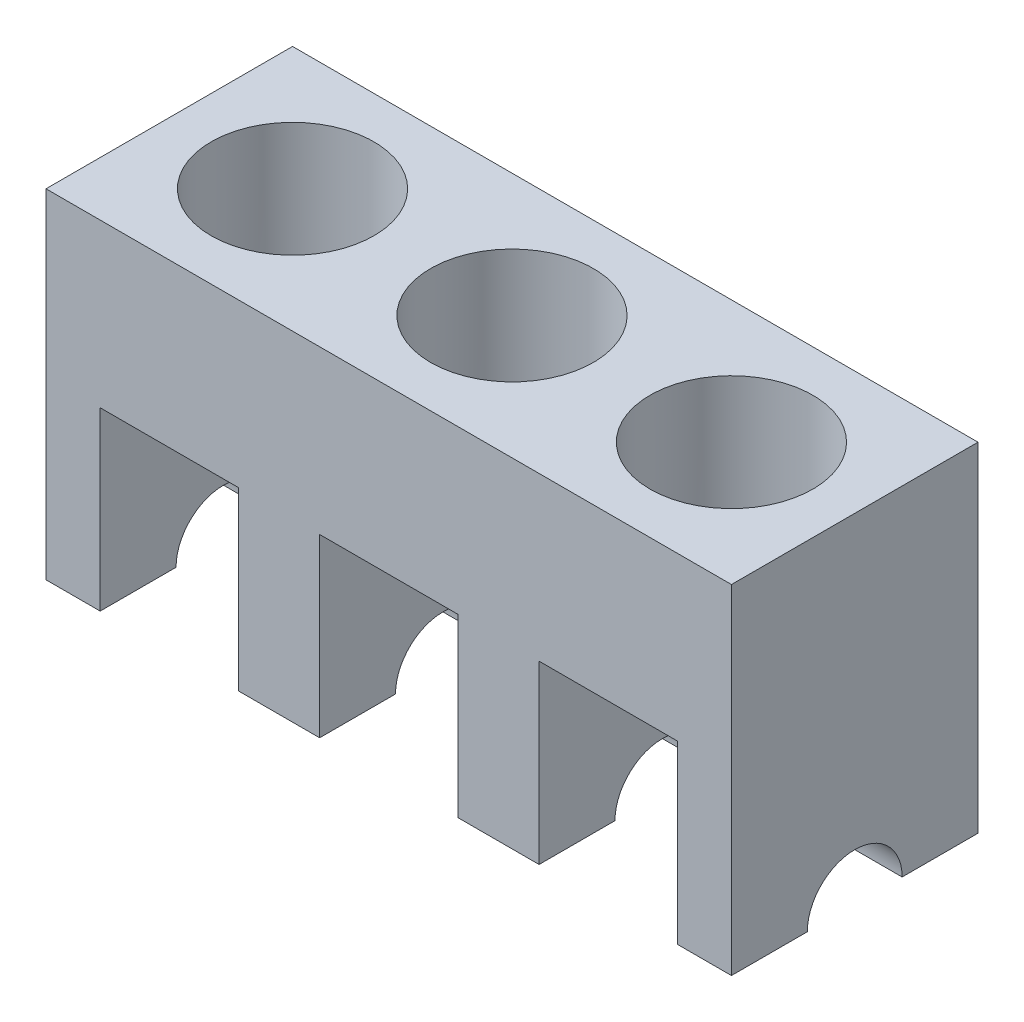
ISO-10303-21;
HEADER;
FILE_DESCRIPTION(('STEP AP214'),'2;1');
FILE_NAME('part.step','',(''),(''),'','','');
FILE_SCHEMA(('AUTOMOTIVE_DESIGN { 1 0 10303 214 1 1 1 1 }'));
ENDSEC;
DATA;
#1=APPLICATION_CONTEXT('core data for automotive mechanical design processes');
#2=APPLICATION_PROTOCOL_DEFINITION('international standard','automotive_design',2000,#1);
#3=PRODUCT_CONTEXT('',#1,'mechanical');
#4=PRODUCT('Part','Part','',(#3));
#5=PRODUCT_RELATED_PRODUCT_CATEGORY('part','',(#4));
#6=PRODUCT_DEFINITION_FORMATION('','',#4);
#7=PRODUCT_DEFINITION_CONTEXT('part definition',#1,'design');
#8=PRODUCT_DEFINITION('design','',#6,#7);
#9=PRODUCT_DEFINITION_SHAPE('','',#8);
#10=(LENGTH_UNIT() NAMED_UNIT(*) SI_UNIT(.MILLI.,.METRE.));
#11=(NAMED_UNIT(*) PLANE_ANGLE_UNIT() SI_UNIT($,.RADIAN.));
#12=(NAMED_UNIT(*) SI_UNIT($,.STERADIAN.) SOLID_ANGLE_UNIT());
#13=UNCERTAINTY_MEASURE_WITH_UNIT(LENGTH_MEASURE(1.E-05),#10,'distance_accuracy_value','');
#14=(GEOMETRIC_REPRESENTATION_CONTEXT(3) GLOBAL_UNCERTAINTY_ASSIGNED_CONTEXT((#13)) GLOBAL_UNIT_ASSIGNED_CONTEXT((#10,
#11,#12)) REPRESENTATION_CONTEXT('',''));
#15=CARTESIAN_POINT('',(0.,0.,0.));
#16=DIRECTION('',(0.,0.,1.));
#17=DIRECTION('',(1.,0.,0.));
#18=AXIS2_PLACEMENT_3D('',#15,#16,#17);
#19=CARTESIAN_POINT('',(-106.5,2.5,45.5));
#20=DIRECTION('',(0.,1.,0.));
#21=DIRECTION('',(-1.,0.,0.));
#22=AXIS2_PLACEMENT_3D('',#19,#20,#21);
#23=PLANE('',#22);
#24=DIRECTION('',(0.,0.,-1.));
#25=VECTOR('',#24,1.);
#26=CARTESIAN_POINT('',(-106.5,2.5,45.5));
#27=LINE('',#26,#25);
#28=CARTESIAN_POINT('',(-106.5,2.5,45.5));
#29=VERTEX_POINT('',#28);
#30=CARTESIAN_POINT('',(-106.5,2.5,15.8981917210732));
#31=VERTEX_POINT('',#30);
#32=EDGE_CURVE('E322',#29,#31,#27,.T.);
#33=ORIENTED_EDGE('',*,*,#32,.T.);
#34=CARTESIAN_POINT('',(-80.9999999999999,2.5,0.));
#35=DIRECTION('',(0.,1.,0.));
#36=DIRECTION('',(-1.,0.,0.));
#37=AXIS2_PLACEMENT_3D('',#34,#35,#36);
#38=CIRCLE('',#37,30.05);
#39=CARTESIAN_POINT('',(-55.4999999999999,2.5,15.8981917210731));
#40=VERTEX_POINT('',#39);
#41=EDGE_CURVE('E318',#31,#40,#38,.T.);
#42=ORIENTED_EDGE('',*,*,#41,.T.);
#43=DIRECTION('',(0.,0.,-1.));
#44=VECTOR('',#43,1.);
#45=CARTESIAN_POINT('',(-55.4999999999999,2.5,45.5));
#46=LINE('',#45,#44);
#47=CARTESIAN_POINT('',(-55.4999999999999,2.5,45.5));
#48=VERTEX_POINT('',#47);
#49=EDGE_CURVE('E314',#48,#40,#46,.T.);
#50=ORIENTED_EDGE('',*,*,#49,.F.);
#51=DIRECTION('',(1.,0.,0.));
#52=VECTOR('',#51,1.);
#53=CARTESIAN_POINT('',(-106.5,2.5,45.5));
#54=LINE('',#53,#52);
#55=EDGE_CURVE('E397',#29,#48,#54,.T.);
#56=ORIENTED_EDGE('',*,*,#55,.F.);
#57=EDGE_LOOP('',(#33,#42,#50,#56));
#58=FACE_BOUND('',#57,.T.);
#59=ADVANCED_FACE('F39',(#58),#23,.F.);
#60=CARTESIAN_POINT('',(-25.4999999999999,2.5,45.5));
#61=DIRECTION('',(0.,1.,0.));
#62=DIRECTION('',(0.,0.,1.));
#63=AXIS2_PLACEMENT_3D('',#60,#61,#62);
#64=PLANE('',#63);
#65=DIRECTION('',(0.,0.,-1.));
#66=VECTOR('',#65,1.);
#67=CARTESIAN_POINT('',(25.5000000000001,2.5,45.5));
#68=LINE('',#67,#66);
#69=CARTESIAN_POINT('',(25.5000000000001,2.5,-15.898191721073));
#70=VERTEX_POINT('',#69);
#71=CARTESIAN_POINT('',(25.5000000000001,2.5,-45.5));
#72=VERTEX_POINT('',#71);
#73=EDGE_CURVE('E484',#70,#72,#68,.T.);
#74=ORIENTED_EDGE('',*,*,#73,.F.);
#75=CARTESIAN_POINT('',(0.,2.5,0.));
#76=DIRECTION('',(0.,1.,0.));
#77=DIRECTION('',(0.,0.,1.));
#78=AXIS2_PLACEMENT_3D('',#75,#76,#77);
#79=CIRCLE('',#78,30.05);
#80=CARTESIAN_POINT('',(-25.4999999999999,2.5,-15.8981917210733));
#81=VERTEX_POINT('',#80);
#82=EDGE_CURVE('E617',#70,#81,#79,.T.);
#83=ORIENTED_EDGE('',*,*,#82,.T.);
#84=DIRECTION('',(0.,0.,-1.));
#85=VECTOR('',#84,1.);
#86=CARTESIAN_POINT('',(-25.4999999999999,2.5,45.5));
#87=LINE('',#86,#85);
#88=CARTESIAN_POINT('',(-25.4999999999999,2.5,-45.5));
#89=VERTEX_POINT('',#88);
#90=EDGE_CURVE('E487',#81,#89,#87,.T.);
#91=ORIENTED_EDGE('',*,*,#90,.T.);
#92=DIRECTION('',(1.,0.,0.));
#93=VECTOR('',#92,1.);
#94=CARTESIAN_POINT('',(-25.4999999999999,2.5,-45.5));
#95=LINE('',#94,#93);
#96=EDGE_CURVE('E441',#89,#72,#95,.T.);
#97=ORIENTED_EDGE('',*,*,#96,.T.);
#98=EDGE_LOOP('',(#74,#83,#91,#97));
#99=FACE_BOUND('',#98,.T.);
#100=ADVANCED_FACE('F621',(#99),#64,.F.);
#101=CARTESIAN_POINT('',(55.5000000000001,2.5,45.5));
#102=DIRECTION('',(0.,1.,0.));
#103=DIRECTION('',(0.,0.,1.));
#104=AXIS2_PLACEMENT_3D('',#101,#102,#103);
#105=PLANE('',#104);
#106=DIRECTION('',(0.,0.,-1.));
#107=VECTOR('',#106,1.);
#108=CARTESIAN_POINT('',(106.5,2.5,45.5));
#109=LINE('',#108,#107);
#110=CARTESIAN_POINT('',(106.5,2.5,-15.8981917210732));
#111=VERTEX_POINT('',#110);
#112=CARTESIAN_POINT('',(106.5,2.5,-45.5));
#113=VERTEX_POINT('',#112);
#114=EDGE_CURVE('E473',#111,#113,#109,.T.);
#115=ORIENTED_EDGE('',*,*,#114,.F.);
#116=CARTESIAN_POINT('',(81.0000000000001,2.5,0.));
#117=DIRECTION('',(0.,1.,0.));
#118=DIRECTION('',(0.,0.,1.));
#119=AXIS2_PLACEMENT_3D('',#116,#117,#118);
#120=CIRCLE('',#119,30.05);
#121=CARTESIAN_POINT('',(55.5000000000001,2.5,-15.8981917210732));
#122=VERTEX_POINT('',#121);
#123=EDGE_CURVE('E601',#111,#122,#120,.T.);
#124=ORIENTED_EDGE('',*,*,#123,.T.);
#125=DIRECTION('',(0.,0.,-1.));
#126=VECTOR('',#125,1.);
#127=CARTESIAN_POINT('',(55.5000000000001,2.5,45.5));
#128=LINE('',#127,#126);
#129=CARTESIAN_POINT('',(55.5000000000001,2.5,-45.5));
#130=VERTEX_POINT('',#129);
#131=EDGE_CURVE('E471',#122,#130,#128,.T.);
#132=ORIENTED_EDGE('',*,*,#131,.T.);
#133=DIRECTION('',(1.,0.,0.));
#134=VECTOR('',#133,1.);
#135=CARTESIAN_POINT('',(55.5000000000001,2.5,-45.5));
#136=LINE('',#135,#134);
#137=EDGE_CURVE('E457',#130,#113,#136,.T.);
#138=ORIENTED_EDGE('',*,*,#137,.T.);
#139=EDGE_LOOP('',(#115,#124,#132,#138));
#140=FACE_BOUND('',#139,.T.);
#141=ADVANCED_FACE('F655',(#140),#105,.F.);
#142=CARTESIAN_POINT('',(-126.5,-62.5,45.5));
#143=DIRECTION('',(0.,1.,0.));
#144=DIRECTION('',(0.,0.,1.));
#145=AXIS2_PLACEMENT_3D('',#142,#143,#144);
#146=PLANE('',#145);
#147=DIRECTION('',(0.,0.,-1.));
#148=VECTOR('',#147,1.);
#149=CARTESIAN_POINT('',(-126.5,-62.5,45.5));
#150=LINE('',#149,#148);
#151=CARTESIAN_POINT('',(-126.5,-62.5,45.5));
#152=VERTEX_POINT('',#151);
#153=CARTESIAN_POINT('',(-126.5,-62.5,17.5));
#154=VERTEX_POINT('',#153);
#155=EDGE_CURVE('E508',#152,#154,#150,.T.);
#156=ORIENTED_EDGE('',*,*,#155,.T.);
#157=DIRECTION('',(1.,0.,0.));
#158=VECTOR('',#157,1.);
#159=CARTESIAN_POINT('',(-126.5,-62.5,17.5));
#160=LINE('',#159,#158);
#161=CARTESIAN_POINT('',(-106.5,-62.5,17.5));
#162=VERTEX_POINT('',#161);
#163=EDGE_CURVE('E379',#154,#162,#160,.T.);
#164=ORIENTED_EDGE('',*,*,#163,.T.);
#165=DIRECTION('',(0.,0.,-1.));
#166=VECTOR('',#165,1.);
#167=CARTESIAN_POINT('',(-106.5,-62.5,45.5));
#168=LINE('',#167,#166);
#169=CARTESIAN_POINT('',(-106.5,-62.5,45.5));
#170=VERTEX_POINT('',#169);
#171=EDGE_CURVE('E507',#170,#162,#168,.T.);
#172=ORIENTED_EDGE('',*,*,#171,.F.);
#173=DIRECTION('',(1.,0.,0.));
#174=VECTOR('',#173,1.);
#175=CARTESIAN_POINT('',(-126.5,-62.5,45.5));
#176=LINE('',#175,#174);
#177=EDGE_CURVE('E395',#152,#170,#176,.T.);
#178=ORIENTED_EDGE('',*,*,#177,.F.);
#179=EDGE_LOOP('',(#156,#164,#172,#178));
#180=FACE_BOUND('',#179,.T.);
#181=ADVANCED_FACE('F558',(#180),#146,.F.);
#182=CARTESIAN_POINT('',(-55.4999999999999,-62.5,45.5));
#183=DIRECTION('',(0.,1.,0.));
#184=DIRECTION('',(-1.,0.,0.));
#185=AXIS2_PLACEMENT_3D('',#182,#183,#184);
#186=PLANE('',#185);
#187=DIRECTION('',(0.,0.,-1.));
#188=VECTOR('',#187,1.);
#189=CARTESIAN_POINT('',(-55.4999999999999,-62.5,45.5));
#190=LINE('',#189,#188);
#191=CARTESIAN_POINT('',(-55.4999999999999,-62.5,45.5));
#192=VERTEX_POINT('',#191);
#193=CARTESIAN_POINT('',(-55.4999999999999,-62.5,17.5));
#194=VERTEX_POINT('',#193);
#195=EDGE_CURVE('E499',#192,#194,#190,.T.);
#196=ORIENTED_EDGE('',*,*,#195,.T.);
#197=DIRECTION('',(1.,0.,0.));
#198=VECTOR('',#197,1.);
#199=CARTESIAN_POINT('',(-126.5,-62.5,17.5));
#200=LINE('',#199,#198);
#201=CARTESIAN_POINT('',(-25.4999999999999,-62.5,17.5));
#202=VERTEX_POINT('',#201);
#203=EDGE_CURVE('E366',#194,#202,#200,.T.);
#204=ORIENTED_EDGE('',*,*,#203,.T.);
#205=DIRECTION('',(0.,0.,-1.));
#206=VECTOR('',#205,1.);
#207=CARTESIAN_POINT('',(-25.4999999999999,-62.5,45.5));
#208=LINE('',#207,#206);
#209=CARTESIAN_POINT('',(-25.4999999999999,-62.5,45.5));
#210=VERTEX_POINT('',#209);
#211=EDGE_CURVE('E493',#210,#202,#208,.T.);
#212=ORIENTED_EDGE('',*,*,#211,.F.);
#213=DIRECTION('',(1.,0.,0.));
#214=VECTOR('',#213,1.);
#215=CARTESIAN_POINT('',(-55.4999999999999,-62.5,45.5));
#216=LINE('',#215,#214);
#217=EDGE_CURVE('E398',#192,#210,#216,.T.);
#218=ORIENTED_EDGE('',*,*,#217,.F.);
#219=EDGE_LOOP('',(#196,#204,#212,#218));
#220=FACE_BOUND('',#219,.T.);
#221=ADVANCED_FACE('F567',(#220),#186,.F.);
#222=CARTESIAN_POINT('',(25.5000000000001,-62.5,45.5));
#223=DIRECTION('',(0.,1.,0.));
#224=DIRECTION('',(0.,0.,1.));
#225=AXIS2_PLACEMENT_3D('',#222,#223,#224);
#226=PLANE('',#225);
#227=DIRECTION('',(0.,0.,-1.));
#228=VECTOR('',#227,1.);
#229=CARTESIAN_POINT('',(25.5000000000001,-62.5,45.5));
#230=LINE('',#229,#228);
#231=CARTESIAN_POINT('',(25.5000000000001,-62.5,45.5));
#232=VERTEX_POINT('',#231);
#233=CARTESIAN_POINT('',(25.5000000000001,-62.5,17.5));
#234=VERTEX_POINT('',#233);
#235=EDGE_CURVE('E485',#232,#234,#230,.T.);
#236=ORIENTED_EDGE('',*,*,#235,.T.);
#237=DIRECTION('',(1.,0.,0.));
#238=VECTOR('',#237,1.);
#239=CARTESIAN_POINT('',(-126.5,-62.5,17.5));
#240=LINE('',#239,#238);
#241=CARTESIAN_POINT('',(55.5000000000001,-62.5,17.5));
#242=VERTEX_POINT('',#241);
#243=EDGE_CURVE('E357',#234,#242,#240,.T.);
#244=ORIENTED_EDGE('',*,*,#243,.T.);
#245=DIRECTION('',(0.,0.,-1.));
#246=VECTOR('',#245,1.);
#247=CARTESIAN_POINT('',(55.5000000000001,-62.5,45.5));
#248=LINE('',#247,#246);
#249=CARTESIAN_POINT('',(55.5000000000001,-62.5,45.5));
#250=VERTEX_POINT('',#249);
#251=EDGE_CURVE('E476',#250,#242,#248,.T.);
#252=ORIENTED_EDGE('',*,*,#251,.F.);
#253=DIRECTION('',(1.,0.,0.));
#254=VECTOR('',#253,1.);
#255=CARTESIAN_POINT('',(25.5000000000001,-62.5,45.5));
#256=LINE('',#255,#254);
#257=EDGE_CURVE('E407',#232,#250,#256,.T.);
#258=ORIENTED_EDGE('',*,*,#257,.F.);
#259=EDGE_LOOP('',(#236,#244,#252,#258));
#260=FACE_BOUND('',#259,.T.);
#261=ADVANCED_FACE('F586',(#260),#226,.F.);
#262=CARTESIAN_POINT('',(106.5,-62.5,45.5));
#263=DIRECTION('',(0.,1.,0.));
#264=DIRECTION('',(0.,0.,1.));
#265=AXIS2_PLACEMENT_3D('',#262,#263,#264);
#266=PLANE('',#265);
#267=DIRECTION('',(0.,0.,-1.));
#268=VECTOR('',#267,1.);
#269=CARTESIAN_POINT('',(106.5,-62.5,45.5));
#270=LINE('',#269,#268);
#271=CARTESIAN_POINT('',(106.5,-62.5,45.5));
#272=VERTEX_POINT('',#271);
#273=CARTESIAN_POINT('',(106.5,-62.5,17.5));
#274=VERTEX_POINT('',#273);
#275=EDGE_CURVE('E469',#272,#274,#270,.T.);
#276=ORIENTED_EDGE('',*,*,#275,.T.);
#277=DIRECTION('',(1.,0.,0.));
#278=VECTOR('',#277,1.);
#279=CARTESIAN_POINT('',(-126.5,-62.5,17.5));
#280=LINE('',#279,#278);
#281=CARTESIAN_POINT('',(126.5,-62.5,17.5));
#282=VERTEX_POINT('',#281);
#283=EDGE_CURVE('E278',#274,#282,#280,.T.);
#284=ORIENTED_EDGE('',*,*,#283,.T.);
#285=DIRECTION('',(0.,0.,-1.));
#286=VECTOR('',#285,1.);
#287=CARTESIAN_POINT('',(126.5,-62.5,45.5));
#288=LINE('',#287,#286);
#289=CARTESIAN_POINT('',(126.5,-62.5,45.5));
#290=VERTEX_POINT('',#289);
#291=EDGE_CURVE('E463',#290,#282,#288,.T.);
#292=ORIENTED_EDGE('',*,*,#291,.F.);
#293=DIRECTION('',(1.,0.,0.));
#294=VECTOR('',#293,1.);
#295=CARTESIAN_POINT('',(106.5,-62.5,45.5));
#296=LINE('',#295,#294);
#297=EDGE_CURVE('E418',#272,#290,#296,.T.);
#298=ORIENTED_EDGE('',*,*,#297,.F.);
#299=EDGE_LOOP('',(#276,#284,#292,#298));
#300=FACE_BOUND('',#299,.T.);
#301=ADVANCED_FACE('F521',(#300),#266,.F.);
#302=CARTESIAN_POINT('',(126.5,-62.5,45.5));
#303=DIRECTION('',(-1.,0.,0.));
#304=DIRECTION('',(0.,0.,1.));
#305=AXIS2_PLACEMENT_3D('',#302,#303,#304);
#306=PLANE('',#305);
#307=ORIENTED_EDGE('',*,*,#291,.T.);
#308=CARTESIAN_POINT('',(126.5,-62.5,0.));
#309=DIRECTION('',(1.,0.,0.));
#310=DIRECTION('',(0.,0.,-1.));
#311=AXIS2_PLACEMENT_3D('',#308,#309,#310);
#312=CIRCLE('',#311,17.5);
#313=CARTESIAN_POINT('',(126.5,-62.5,-17.5));
#314=VERTEX_POINT('',#313);
#315=EDGE_CURVE('E337',#314,#282,#312,.T.);
#316=ORIENTED_EDGE('',*,*,#315,.F.);
#317=CARTESIAN_POINT('',(126.5,-62.5,-45.5));
#318=VERTEX_POINT('',#317);
#319=EDGE_CURVE('E416',#314,#318,#288,.T.);
#320=ORIENTED_EDGE('',*,*,#319,.T.);
#321=DIRECTION('',(0.,1.,0.));
#322=VECTOR('',#321,1.);
#323=CARTESIAN_POINT('',(126.5,-62.5,-45.5));
#324=LINE('',#323,#322);
#325=CARTESIAN_POINT('',(126.5,62.5,-45.5));
#326=VERTEX_POINT('',#325);
#327=EDGE_CURVE('E382',#318,#326,#324,.T.);
#328=ORIENTED_EDGE('',*,*,#327,.T.);
#329=DIRECTION('',(0.,0.,-1.));
#330=VECTOR('',#329,1.);
#331=CARTESIAN_POINT('',(126.5,62.5,45.5));
#332=LINE('',#331,#330);
#333=CARTESIAN_POINT('',(126.5,62.5,45.5));
#334=VERTEX_POINT('',#333);
#335=EDGE_CURVE('E516',#334,#326,#332,.T.);
#336=ORIENTED_EDGE('',*,*,#335,.F.);
#337=DIRECTION('',(0.,1.,0.));
#338=VECTOR('',#337,1.);
#339=CARTESIAN_POINT('',(126.5,-62.5,45.5));
#340=LINE('',#339,#338);
#341=EDGE_CURVE('E383',#290,#334,#340,.T.);
#342=ORIENTED_EDGE('',*,*,#341,.F.);
#343=EDGE_LOOP('',(#307,#316,#320,#328,#336,#342));
#344=FACE_BOUND('',#343,.T.);
#345=ADVANCED_FACE('F41',(#344),#306,.F.);
#346=CARTESIAN_POINT('',(-126.5,62.5,45.5));
#347=DIRECTION('',(0.,-1.,0.));
#348=DIRECTION('',(0.,0.,-1.));
#349=AXIS2_PLACEMENT_3D('',#346,#347,#348);
#350=PLANE('',#349);
#351=CARTESIAN_POINT('',(-80.9999999999999,62.5,0.));
#352=DIRECTION('',(0.,1.,0.));
#353=DIRECTION('',(0.,0.,1.));
#354=AXIS2_PLACEMENT_3D('',#351,#352,#353);
#355=CIRCLE('',#354,30.05);
#356=CARTESIAN_POINT('',(-80.9999999999999,62.5,30.05));
#357=VERTEX_POINT('',#356);
#358=EDGE_CURVE('E634',#357,#357,#355,.T.);
#359=ORIENTED_EDGE('',*,*,#358,.F.);
#360=EDGE_LOOP('',(#359));
#361=FACE_BOUND('',#360,.T.);
#362=CARTESIAN_POINT('',(0.,62.5,0.));
#363=DIRECTION('',(0.,1.,0.));
#364=DIRECTION('',(0.,0.,1.));
#365=AXIS2_PLACEMENT_3D('',#362,#363,#364);
#366=CIRCLE('',#365,30.05);
#367=CARTESIAN_POINT('',(0.,62.5,30.05));
#368=VERTEX_POINT('',#367);
#369=EDGE_CURVE('E287',#368,#368,#366,.T.);
#370=ORIENTED_EDGE('',*,*,#369,.F.);
#371=EDGE_LOOP('',(#370));
#372=FACE_BOUND('',#371,.T.);
#373=CARTESIAN_POINT('',(81.0000000000001,62.5,0.));
#374=DIRECTION('',(0.,1.,0.));
#375=DIRECTION('',(0.,0.,1.));
#376=AXIS2_PLACEMENT_3D('',#373,#374,#375);
#377=CIRCLE('',#376,30.05);
#378=CARTESIAN_POINT('',(81.0000000000001,62.5,30.05));
#379=VERTEX_POINT('',#378);
#380=EDGE_CURVE('E644',#379,#379,#377,.T.);
#381=ORIENTED_EDGE('',*,*,#380,.F.);
#382=EDGE_LOOP('',(#381));
#383=FACE_BOUND('',#382,.T.);
#384=DIRECTION('',(-1.,0.,0.));
#385=VECTOR('',#384,1.);
#386=CARTESIAN_POINT('',(-126.5,62.5,-45.5));
#387=LINE('',#386,#385);
#388=CARTESIAN_POINT('',(-126.5,62.5,-45.5));
#389=VERTEX_POINT('',#388);
#390=EDGE_CURVE('E423',#326,#389,#387,.T.);
#391=ORIENTED_EDGE('',*,*,#390,.T.);
#392=DIRECTION('',(0.,0.,-1.));
#393=VECTOR('',#392,1.);
#394=CARTESIAN_POINT('',(-126.5,62.5,45.5));
#395=LINE('',#394,#393);
#396=CARTESIAN_POINT('',(-126.5,62.5,45.5));
#397=VERTEX_POINT('',#396);
#398=EDGE_CURVE('E511',#397,#389,#395,.T.);
#399=ORIENTED_EDGE('',*,*,#398,.F.);
#400=DIRECTION('',(-1.,0.,0.));
#401=VECTOR('',#400,1.);
#402=CARTESIAN_POINT('',(-126.5,62.5,45.5));
#403=LINE('',#402,#401);
#404=EDGE_CURVE('E390',#334,#397,#403,.T.);
#405=ORIENTED_EDGE('',*,*,#404,.F.);
#406=ORIENTED_EDGE('',*,*,#335,.T.);
#407=EDGE_LOOP('',(#391,#399,#405,#406));
#408=FACE_BOUND('',#407,.T.);
#409=ADVANCED_FACE('F548',(#361,#372,#383,#408),#350,.F.);
#410=CARTESIAN_POINT('',(-126.5,-62.5,45.5));
#411=DIRECTION('',(1.,0.,0.));
#412=DIRECTION('',(0.,0.,-1.));
#413=AXIS2_PLACEMENT_3D('',#410,#411,#412);
#414=PLANE('',#413);
#415=CARTESIAN_POINT('',(-126.5,-62.5,-17.5));
#416=VERTEX_POINT('',#415);
#417=CARTESIAN_POINT('',(-126.5,-62.5,-45.5));
#418=VERTEX_POINT('',#417);
#419=EDGE_CURVE('E506',#416,#418,#150,.T.);
#420=ORIENTED_EDGE('',*,*,#419,.F.);
#421=CARTESIAN_POINT('',(-126.5,-62.5,0.));
#422=DIRECTION('',(1.,0.,0.));
#423=DIRECTION('',(0.,0.,-1.));
#424=AXIS2_PLACEMENT_3D('',#421,#422,#423);
#425=CIRCLE('',#424,17.5);
#426=EDGE_CURVE('E345',#416,#154,#425,.T.);
#427=ORIENTED_EDGE('',*,*,#426,.T.);
#428=ORIENTED_EDGE('',*,*,#155,.F.);
#429=DIRECTION('',(0.,-1.,0.));
#430=VECTOR('',#429,1.);
#431=CARTESIAN_POINT('',(-126.5,-62.5,45.5));
#432=LINE('',#431,#430);
#433=EDGE_CURVE('E388',#397,#152,#432,.T.);
#434=ORIENTED_EDGE('',*,*,#433,.F.);
#435=ORIENTED_EDGE('',*,*,#398,.T.);
#436=DIRECTION('',(0.,-1.,0.));
#437=VECTOR('',#436,1.);
#438=CARTESIAN_POINT('',(-126.5,-62.5,-45.5));
#439=LINE('',#438,#437);
#440=EDGE_CURVE('E421',#389,#418,#439,.T.);
#441=ORIENTED_EDGE('',*,*,#440,.T.);
#442=EDGE_LOOP('',(#420,#427,#428,#434,#435,#441));
#443=FACE_BOUND('',#442,.T.);
#444=ADVANCED_FACE('F551',(#443),#414,.F.);
#445=CARTESIAN_POINT('',(-106.5,-62.5,-17.5));
#446=VERTEX_POINT('',#445);
#447=CARTESIAN_POINT('',(-106.5,-62.5,-45.5));
#448=VERTEX_POINT('',#447);
#449=EDGE_CURVE('E504',#446,#448,#168,.T.);
#450=ORIENTED_EDGE('',*,*,#449,.F.);
#451=DIRECTION('',(1.,0.,0.));
#452=VECTOR('',#451,1.);
#453=CARTESIAN_POINT('',(-126.5,-62.5,-17.5));
#454=LINE('',#453,#452);
#455=EDGE_CURVE('E380',#446,#416,#454,.F.);
#456=ORIENTED_EDGE('',*,*,#455,.T.);
#457=ORIENTED_EDGE('',*,*,#419,.T.);
#458=DIRECTION('',(1.,0.,0.));
#459=VECTOR('',#458,1.);
#460=CARTESIAN_POINT('',(-126.5,-62.5,-45.5));
#461=LINE('',#460,#459);
#462=EDGE_CURVE('E426',#418,#448,#461,.T.);
#463=ORIENTED_EDGE('',*,*,#462,.T.);
#464=EDGE_LOOP('',(#450,#456,#457,#463));
#465=FACE_BOUND('',#464,.T.);
#466=ADVANCED_FACE('F687',(#465),#146,.F.);
#467=CARTESIAN_POINT('',(-106.5,-62.5,45.5));
#468=DIRECTION('',(-1.,0.,0.));
#469=DIRECTION('',(0.,-1.,0.));
#470=AXIS2_PLACEMENT_3D('',#467,#468,#469);
#471=PLANE('',#470);
#472=DIRECTION('',(0.,0.,-1.));
#473=VECTOR('',#472,1.);
#474=CARTESIAN_POINT('',(-106.5,-18.5,45.5));
#475=LINE('',#474,#473);
#476=CARTESIAN_POINT('',(-106.5,-18.5,15.8981917210732));
#477=VERTEX_POINT('',#476);
#478=CARTESIAN_POINT('',(-106.5,-18.5,-15.8981917210732));
#479=VERTEX_POINT('',#478);
#480=EDGE_CURVE('E326',#477,#479,#475,.T.);
#481=ORIENTED_EDGE('',*,*,#480,.F.);
#482=DIRECTION('',(0.,1.,0.));
#483=VECTOR('',#482,1.);
#484=CARTESIAN_POINT('',(-106.5,-18.5,15.8981917210732));
#485=LINE('',#484,#483);
#486=EDGE_CURVE('E324',#477,#31,#485,.T.);
#487=ORIENTED_EDGE('',*,*,#486,.T.);
#488=ORIENTED_EDGE('',*,*,#32,.F.);
#489=DIRECTION('',(0.,1.,0.));
#490=VECTOR('',#489,1.);
#491=CARTESIAN_POINT('',(-106.5,-62.5,45.5));
#492=LINE('',#491,#490);
#493=EDGE_CURVE('E393',#170,#29,#492,.T.);
#494=ORIENTED_EDGE('',*,*,#493,.F.);
#495=ORIENTED_EDGE('',*,*,#171,.T.);
#496=CARTESIAN_POINT('',(-106.5,-62.5,0.));
#497=DIRECTION('',(-1.,0.,0.));
#498=DIRECTION('',(0.,-1.,0.));
#499=AXIS2_PLACEMENT_3D('',#496,#497,#498);
#500=CIRCLE('',#499,17.5);
#501=EDGE_CURVE('E372',#162,#446,#500,.T.);
#502=ORIENTED_EDGE('',*,*,#501,.T.);
#503=ORIENTED_EDGE('',*,*,#449,.T.);
#504=DIRECTION('',(0.,1.,0.));
#505=VECTOR('',#504,1.);
#506=CARTESIAN_POINT('',(-106.5,-62.5,-45.5));
#507=LINE('',#506,#505);
#508=CARTESIAN_POINT('',(-106.5,2.5,-45.5));
#509=VERTEX_POINT('',#508);
#510=EDGE_CURVE('E427',#448,#509,#507,.T.);
#511=ORIENTED_EDGE('',*,*,#510,.T.);
#512=CARTESIAN_POINT('',(-106.5,2.5,-15.8981917210732));
#513=VERTEX_POINT('',#512);
#514=EDGE_CURVE('E502',#513,#509,#27,.T.);
#515=ORIENTED_EDGE('',*,*,#514,.F.);
#516=DIRECTION('',(0.,1.,0.));
#517=VECTOR('',#516,1.);
#518=CARTESIAN_POINT('',(-106.5,-18.5,-15.8981917210732));
#519=LINE('',#518,#517);
#520=EDGE_CURVE('E334',#513,#479,#519,.F.);
#521=ORIENTED_EDGE('',*,*,#520,.T.);
#522=EDGE_LOOP('',(#481,#487,#488,#494,#495,#502,#503,#511,#515,#521));
#523=FACE_BOUND('',#522,.T.);
#524=ADVANCED_FACE('F559',(#523),#471,.F.);
#525=CARTESIAN_POINT('',(-55.4999999999999,2.5,-15.8981917210731));
#526=VERTEX_POINT('',#525);
#527=CARTESIAN_POINT('',(-55.4999999999999,2.5,-45.5));
#528=VERTEX_POINT('',#527);
#529=EDGE_CURVE('E501',#526,#528,#46,.T.);
#530=ORIENTED_EDGE('',*,*,#529,.F.);
#531=EDGE_CURVE('E327',#526,#513,#38,.T.);
#532=ORIENTED_EDGE('',*,*,#531,.T.);
#533=ORIENTED_EDGE('',*,*,#514,.T.);
#534=DIRECTION('',(1.,0.,0.));
#535=VECTOR('',#534,1.);
#536=CARTESIAN_POINT('',(-106.5,2.5,-45.5));
#537=LINE('',#536,#535);
#538=EDGE_CURVE('E435',#509,#528,#537,.T.);
#539=ORIENTED_EDGE('',*,*,#538,.T.);
#540=EDGE_LOOP('',(#530,#532,#533,#539));
#541=FACE_BOUND('',#540,.T.);
#542=ADVANCED_FACE('F675',(#541),#23,.F.);
#543=CARTESIAN_POINT('',(-55.4999999999999,2.5,45.5));
#544=DIRECTION('',(1.,0.,0.));
#545=DIRECTION('',(0.,1.,0.));
#546=AXIS2_PLACEMENT_3D('',#543,#544,#545);
#547=PLANE('',#546);
#548=DIRECTION('',(0.,0.,1.));
#549=VECTOR('',#548,1.);
#550=CARTESIAN_POINT('',(-55.4999999999999,-18.5,45.5));
#551=LINE('',#550,#549);
#552=CARTESIAN_POINT('',(-55.4999999999999,-18.5,-15.8981917210731));
#553=VERTEX_POINT('',#552);
#554=CARTESIAN_POINT('',(-55.4999999999999,-18.5,15.8981917210731));
#555=VERTEX_POINT('',#554);
#556=EDGE_CURVE('E308',#553,#555,#551,.T.);
#557=ORIENTED_EDGE('',*,*,#556,.F.);
#558=DIRECTION('',(0.,1.,0.));
#559=VECTOR('',#558,1.);
#560=CARTESIAN_POINT('',(-55.4999999999999,-18.5,-15.8981917210731));
#561=LINE('',#560,#559);
#562=EDGE_CURVE('E11',#553,#526,#561,.T.);
#563=ORIENTED_EDGE('',*,*,#562,.T.);
#564=ORIENTED_EDGE('',*,*,#529,.T.);
#565=DIRECTION('',(0.,-1.,0.));
#566=VECTOR('',#565,1.);
#567=CARTESIAN_POINT('',(-55.4999999999999,2.5,-45.5));
#568=LINE('',#567,#566);
#569=CARTESIAN_POINT('',(-55.4999999999999,-62.5,-45.5));
#570=VERTEX_POINT('',#569);
#571=EDGE_CURVE('E434',#528,#570,#568,.T.);
#572=ORIENTED_EDGE('',*,*,#571,.T.);
#573=CARTESIAN_POINT('',(-55.4999999999999,-62.5,-17.5));
#574=VERTEX_POINT('',#573);
#575=EDGE_CURVE('E500',#574,#570,#190,.T.);
#576=ORIENTED_EDGE('',*,*,#575,.F.);
#577=CARTESIAN_POINT('',(-55.4999999999999,-62.5,0.));
#578=DIRECTION('',(1.,0.,0.));
#579=DIRECTION('',(0.,1.,0.));
#580=AXIS2_PLACEMENT_3D('',#577,#578,#579);
#581=CIRCLE('',#580,17.5);
#582=EDGE_CURVE('E371',#574,#194,#581,.T.);
#583=ORIENTED_EDGE('',*,*,#582,.T.);
#584=ORIENTED_EDGE('',*,*,#195,.F.);
#585=DIRECTION('',(0.,-1.,0.));
#586=VECTOR('',#585,1.);
#587=CARTESIAN_POINT('',(-55.4999999999999,2.5,45.5));
#588=LINE('',#587,#586);
#589=EDGE_CURVE('E399',#48,#192,#588,.T.);
#590=ORIENTED_EDGE('',*,*,#589,.F.);
#591=ORIENTED_EDGE('',*,*,#49,.T.);
#592=DIRECTION('',(0.,1.,0.));
#593=VECTOR('',#592,1.);
#594=CARTESIAN_POINT('',(-55.4999999999999,-18.5,15.8981917210731));
#595=LINE('',#594,#593);
#596=EDGE_CURVE('E50',#40,#555,#595,.F.);
#597=ORIENTED_EDGE('',*,*,#596,.T.);
#598=EDGE_LOOP('',(#557,#563,#564,#572,#576,#583,#584,#590,#591,#597));
#599=FACE_BOUND('',#598,.T.);
#600=ADVANCED_FACE('F313',(#599),#547,.F.);
#601=CARTESIAN_POINT('',(-25.4999999999999,-62.5,-17.5));
#602=VERTEX_POINT('',#601);
#603=CARTESIAN_POINT('',(-25.4999999999999,-62.5,-45.5));
#604=VERTEX_POINT('',#603);
#605=EDGE_CURVE('E492',#602,#604,#208,.T.);
#606=ORIENTED_EDGE('',*,*,#605,.F.);
#607=DIRECTION('',(1.,0.,0.));
#608=VECTOR('',#607,1.);
#609=CARTESIAN_POINT('',(-126.5,-62.5,-17.5));
#610=LINE('',#609,#608);
#611=EDGE_CURVE('E364',#602,#574,#610,.F.);
#612=ORIENTED_EDGE('',*,*,#611,.T.);
#613=ORIENTED_EDGE('',*,*,#575,.T.);
#614=DIRECTION('',(1.,0.,0.));
#615=VECTOR('',#614,1.);
#616=CARTESIAN_POINT('',(-55.4999999999999,-62.5,-45.5));
#617=LINE('',#616,#615);
#618=EDGE_CURVE('E437',#570,#604,#617,.T.);
#619=ORIENTED_EDGE('',*,*,#618,.T.);
#620=EDGE_LOOP('',(#606,#612,#613,#619));
#621=FACE_BOUND('',#620,.T.);
#622=ADVANCED_FACE('F684',(#621),#186,.F.);
#623=CARTESIAN_POINT('',(-25.4999999999999,-62.5,45.5));
#624=DIRECTION('',(-1.,0.,0.));
#625=DIRECTION('',(0.,0.,1.));
#626=AXIS2_PLACEMENT_3D('',#623,#624,#625);
#627=PLANE('',#626);
#628=DIRECTION('',(0.,0.,-1.));
#629=VECTOR('',#628,1.);
#630=CARTESIAN_POINT('',(-25.4999999999999,-18.5,45.5));
#631=LINE('',#630,#629);
#632=CARTESIAN_POINT('',(-25.4999999999999,-18.5,15.8981917210733));
#633=VERTEX_POINT('',#632);
#634=CARTESIAN_POINT('',(-25.4999999999999,-18.5,-15.8981917210733));
#635=VERTEX_POINT('',#634);
#636=EDGE_CURVE('E608',#633,#635,#631,.T.);
#637=ORIENTED_EDGE('',*,*,#636,.F.);
#638=DIRECTION('',(0.,1.,0.));
#639=VECTOR('',#638,1.);
#640=CARTESIAN_POINT('',(-25.4999999999999,-18.5,15.8981917210733));
#641=LINE('',#640,#639);
#642=CARTESIAN_POINT('',(-25.4999999999999,2.5,15.8981917210733));
#643=VERTEX_POINT('',#642);
#644=EDGE_CURVE('E614',#633,#643,#641,.T.);
#645=ORIENTED_EDGE('',*,*,#644,.T.);
#646=CARTESIAN_POINT('',(-25.4999999999999,2.5,45.5));
#647=VERTEX_POINT('',#646);
#648=EDGE_CURVE('E489',#647,#643,#87,.T.);
#649=ORIENTED_EDGE('',*,*,#648,.F.);
#650=DIRECTION('',(0.,1.,0.));
#651=VECTOR('',#650,1.);
#652=CARTESIAN_POINT('',(-25.4999999999999,-62.5,45.5));
#653=LINE('',#652,#651);
#654=EDGE_CURVE('E405',#210,#647,#653,.T.);
#655=ORIENTED_EDGE('',*,*,#654,.F.);
#656=ORIENTED_EDGE('',*,*,#211,.T.);
#657=CARTESIAN_POINT('',(-25.4999999999999,-62.5,0.));
#658=DIRECTION('',(-1.,0.,0.));
#659=DIRECTION('',(0.,0.,1.));
#660=AXIS2_PLACEMENT_3D('',#657,#658,#659);
#661=CIRCLE('',#660,17.5);
#662=EDGE_CURVE('E362',#202,#602,#661,.T.);
#663=ORIENTED_EDGE('',*,*,#662,.T.);
#664=ORIENTED_EDGE('',*,*,#605,.T.);
#665=DIRECTION('',(0.,1.,0.));
#666=VECTOR('',#665,1.);
#667=CARTESIAN_POINT('',(-25.4999999999999,-62.5,-45.5));
#668=LINE('',#667,#666);
#669=EDGE_CURVE('E442',#604,#89,#668,.T.);
#670=ORIENTED_EDGE('',*,*,#669,.T.);
#671=ORIENTED_EDGE('',*,*,#90,.F.);
#672=DIRECTION('',(0.,1.,0.));
#673=VECTOR('',#672,1.);
#674=CARTESIAN_POINT('',(-25.4999999999999,-18.5,-15.8981917210733));
#675=LINE('',#674,#673);
#676=EDGE_CURVE('E329',#81,#635,#675,.F.);
#677=ORIENTED_EDGE('',*,*,#676,.T.);
#678=EDGE_LOOP('',(#637,#645,#649,#655,#656,#663,#664,#670,#671,#677));
#679=FACE_BOUND('',#678,.T.);
#680=ADVANCED_FACE('F571',(#679),#627,.F.);
#681=ORIENTED_EDGE('',*,*,#648,.T.);
#682=CARTESIAN_POINT('',(25.5000000000001,2.5,15.898191721073));
#683=VERTEX_POINT('',#682);
#684=EDGE_CURVE('E578',#643,#683,#79,.T.);
#685=ORIENTED_EDGE('',*,*,#684,.T.);
#686=CARTESIAN_POINT('',(25.5000000000001,2.5,45.5));
#687=VERTEX_POINT('',#686);
#688=EDGE_CURVE('E486',#687,#683,#68,.T.);
#689=ORIENTED_EDGE('',*,*,#688,.F.);
#690=DIRECTION('',(1.,0.,0.));
#691=VECTOR('',#690,1.);
#692=CARTESIAN_POINT('',(-25.4999999999999,2.5,45.5));
#693=LINE('',#692,#691);
#694=EDGE_CURVE('E404',#647,#687,#693,.T.);
#695=ORIENTED_EDGE('',*,*,#694,.F.);
#696=EDGE_LOOP('',(#681,#685,#689,#695));
#697=FACE_BOUND('',#696,.T.);
#698=ADVANCED_FACE('F576',(#697),#64,.F.);
#699=CARTESIAN_POINT('',(25.5000000000001,2.5,45.5));
#700=DIRECTION('',(1.,0.,0.));
#701=DIRECTION('',(0.,1.,0.));
#702=AXIS2_PLACEMENT_3D('',#699,#700,#701);
#703=PLANE('',#702);
#704=DIRECTION('',(0.,0.,1.));
#705=VECTOR('',#704,1.);
#706=CARTESIAN_POINT('',(25.5000000000001,-18.5,45.5));
#707=LINE('',#706,#705);
#708=CARTESIAN_POINT('',(25.5000000000001,-18.5,-15.898191721073));
#709=VERTEX_POINT('',#708);
#710=CARTESIAN_POINT('',(25.5000000000001,-18.5,15.898191721073));
#711=VERTEX_POINT('',#710);
#712=EDGE_CURVE('E293',#709,#711,#707,.T.);
#713=ORIENTED_EDGE('',*,*,#712,.F.);
#714=DIRECTION('',(0.,1.,0.));
#715=VECTOR('',#714,1.);
#716=CARTESIAN_POINT('',(25.5000000000001,-18.5,-15.898191721073));
#717=LINE('',#716,#715);
#718=EDGE_CURVE('E304',#709,#70,#717,.T.);
#719=ORIENTED_EDGE('',*,*,#718,.T.);
#720=ORIENTED_EDGE('',*,*,#73,.T.);
#721=DIRECTION('',(0.,-1.,0.));
#722=VECTOR('',#721,1.);
#723=CARTESIAN_POINT('',(25.5000000000001,2.5,-45.5));
#724=LINE('',#723,#722);
#725=CARTESIAN_POINT('',(25.5000000000001,-62.5,-45.5));
#726=VERTEX_POINT('',#725);
#727=EDGE_CURVE('E450',#72,#726,#724,.T.);
#728=ORIENTED_EDGE('',*,*,#727,.T.);
#729=CARTESIAN_POINT('',(25.5000000000001,-62.5,-17.5));
#730=VERTEX_POINT('',#729);
#731=EDGE_CURVE('E481',#730,#726,#230,.T.);
#732=ORIENTED_EDGE('',*,*,#731,.F.);
#733=CARTESIAN_POINT('',(25.5000000000001,-62.5,0.));
#734=DIRECTION('',(1.,0.,0.));
#735=DIRECTION('',(0.,1.,0.));
#736=AXIS2_PLACEMENT_3D('',#733,#734,#735);
#737=CIRCLE('',#736,17.5);
#738=EDGE_CURVE('E356',#730,#234,#737,.T.);
#739=ORIENTED_EDGE('',*,*,#738,.T.);
#740=ORIENTED_EDGE('',*,*,#235,.F.);
#741=DIRECTION('',(0.,-1.,0.));
#742=VECTOR('',#741,1.);
#743=CARTESIAN_POINT('',(25.5000000000001,2.5,45.5));
#744=LINE('',#743,#742);
#745=EDGE_CURVE('E406',#687,#232,#744,.T.);
#746=ORIENTED_EDGE('',*,*,#745,.F.);
#747=ORIENTED_EDGE('',*,*,#688,.T.);
#748=DIRECTION('',(0.,1.,0.));
#749=VECTOR('',#748,1.);
#750=CARTESIAN_POINT('',(25.5000000000001,-18.5,15.898191721073));
#751=LINE('',#750,#749);
#752=EDGE_CURVE('E299',#683,#711,#751,.F.);
#753=ORIENTED_EDGE('',*,*,#752,.T.);
#754=EDGE_LOOP('',(#713,#719,#720,#728,#732,#739,#740,#746,#747,#753));
#755=FACE_BOUND('',#754,.T.);
#756=ADVANCED_FACE('F581',(#755),#703,.F.);
#757=CARTESIAN_POINT('',(55.5000000000001,-62.5,-17.5));
#758=VERTEX_POINT('',#757);
#759=CARTESIAN_POINT('',(55.5000000000001,-62.5,-45.5));
#760=VERTEX_POINT('',#759);
#761=EDGE_CURVE('E480',#758,#760,#248,.T.);
#762=ORIENTED_EDGE('',*,*,#761,.F.);
#763=DIRECTION('',(1.,0.,0.));
#764=VECTOR('',#763,1.);
#765=CARTESIAN_POINT('',(-126.5,-62.5,-17.5));
#766=LINE('',#765,#764);
#767=EDGE_CURVE('E352',#758,#730,#766,.F.);
#768=ORIENTED_EDGE('',*,*,#767,.T.);
#769=ORIENTED_EDGE('',*,*,#731,.T.);
#770=DIRECTION('',(1.,0.,0.));
#771=VECTOR('',#770,1.);
#772=CARTESIAN_POINT('',(25.5000000000001,-62.5,-45.5));
#773=LINE('',#772,#771);
#774=EDGE_CURVE('E449',#726,#760,#773,.T.);
#775=ORIENTED_EDGE('',*,*,#774,.T.);
#776=EDGE_LOOP('',(#762,#768,#769,#775));
#777=FACE_BOUND('',#776,.T.);
#778=ADVANCED_FACE('F656',(#777),#226,.F.);
#779=CARTESIAN_POINT('',(55.5000000000001,-62.5,45.5));
#780=DIRECTION('',(-1.,0.,0.));
#781=DIRECTION('',(0.,0.,1.));
#782=AXIS2_PLACEMENT_3D('',#779,#780,#781);
#783=PLANE('',#782);
#784=DIRECTION('',(0.,0.,-1.));
#785=VECTOR('',#784,1.);
#786=CARTESIAN_POINT('',(55.5000000000001,-18.5,45.5));
#787=LINE('',#786,#785);
#788=CARTESIAN_POINT('',(55.5000000000001,-18.5,15.8981917210732));
#789=VERTEX_POINT('',#788);
#790=CARTESIAN_POINT('',(55.5000000000001,-18.5,-15.8981917210732));
#791=VERTEX_POINT('',#790);
#792=EDGE_CURVE('E597',#789,#791,#787,.T.);
#793=ORIENTED_EDGE('',*,*,#792,.F.);
#794=DIRECTION('',(0.,1.,0.));
#795=VECTOR('',#794,1.);
#796=CARTESIAN_POINT('',(55.5000000000001,-18.5,15.8981917210732));
#797=LINE('',#796,#795);
#798=CARTESIAN_POINT('',(55.5000000000001,2.5,15.8981917210732));
#799=VERTEX_POINT('',#798);
#800=EDGE_CURVE('E594',#789,#799,#797,.T.);
#801=ORIENTED_EDGE('',*,*,#800,.T.);
#802=CARTESIAN_POINT('',(55.5000000000001,2.5,45.5));
#803=VERTEX_POINT('',#802);
#804=EDGE_CURVE('E475',#803,#799,#128,.T.);
#805=ORIENTED_EDGE('',*,*,#804,.F.);
#806=DIRECTION('',(0.,1.,0.));
#807=VECTOR('',#806,1.);
#808=CARTESIAN_POINT('',(55.5000000000001,-62.5,45.5));
#809=LINE('',#808,#807);
#810=EDGE_CURVE('E409',#250,#803,#809,.T.);
#811=ORIENTED_EDGE('',*,*,#810,.F.);
#812=ORIENTED_EDGE('',*,*,#251,.T.);
#813=CARTESIAN_POINT('',(55.5000000000001,-62.5,0.));
#814=DIRECTION('',(-1.,0.,0.));
#815=DIRECTION('',(0.,0.,1.));
#816=AXIS2_PLACEMENT_3D('',#813,#814,#815);
#817=CIRCLE('',#816,17.5);
#818=EDGE_CURVE('E348',#242,#758,#817,.T.);
#819=ORIENTED_EDGE('',*,*,#818,.T.);
#820=ORIENTED_EDGE('',*,*,#761,.T.);
#821=DIRECTION('',(0.,1.,0.));
#822=VECTOR('',#821,1.);
#823=CARTESIAN_POINT('',(55.5000000000001,-62.5,-45.5));
#824=LINE('',#823,#822);
#825=EDGE_CURVE('E454',#760,#130,#824,.T.);
#826=ORIENTED_EDGE('',*,*,#825,.T.);
#827=ORIENTED_EDGE('',*,*,#131,.F.);
#828=DIRECTION('',(0.,1.,0.));
#829=VECTOR('',#828,1.);
#830=CARTESIAN_POINT('',(55.5000000000001,-18.5,-15.8981917210732));
#831=LINE('',#830,#829);
#832=EDGE_CURVE('E604',#122,#791,#831,.F.);
#833=ORIENTED_EDGE('',*,*,#832,.T.);
#834=EDGE_LOOP('',(#793,#801,#805,#811,#812,#819,#820,#826,#827,#833));
#835=FACE_BOUND('',#834,.T.);
#836=ADVANCED_FACE('F592',(#835),#783,.F.);
#837=ORIENTED_EDGE('',*,*,#804,.T.);
#838=CARTESIAN_POINT('',(106.5,2.5,15.8981917210732));
#839=VERTEX_POINT('',#838);
#840=EDGE_CURVE('E598',#799,#839,#120,.T.);
#841=ORIENTED_EDGE('',*,*,#840,.T.);
#842=CARTESIAN_POINT('',(106.5,2.5,45.5));
#843=VERTEX_POINT('',#842);
#844=EDGE_CURVE('E291',#843,#839,#109,.T.);
#845=ORIENTED_EDGE('',*,*,#844,.F.);
#846=DIRECTION('',(1.,0.,0.));
#847=VECTOR('',#846,1.);
#848=CARTESIAN_POINT('',(55.5000000000001,2.5,45.5));
#849=LINE('',#848,#847);
#850=EDGE_CURVE('E415',#803,#843,#849,.T.);
#851=ORIENTED_EDGE('',*,*,#850,.F.);
#852=EDGE_LOOP('',(#837,#841,#845,#851));
#853=FACE_BOUND('',#852,.T.);
#854=ADVANCED_FACE('F600',(#853),#105,.F.);
#855=CARTESIAN_POINT('',(106.5,2.5,45.5));
#856=DIRECTION('',(1.,0.,0.));
#857=DIRECTION('',(0.,1.,0.));
#858=AXIS2_PLACEMENT_3D('',#855,#856,#857);
#859=PLANE('',#858);
#860=DIRECTION('',(0.,0.,1.));
#861=VECTOR('',#860,1.);
#862=CARTESIAN_POINT('',(106.5,-18.5,45.5));
#863=LINE('',#862,#861);
#864=CARTESIAN_POINT('',(106.5,-18.5,-15.8981917210732));
#865=VERTEX_POINT('',#864);
#866=CARTESIAN_POINT('',(106.5,-18.5,15.8981917210732));
#867=VERTEX_POINT('',#866);
#868=EDGE_CURVE('E271',#865,#867,#863,.T.);
#869=ORIENTED_EDGE('',*,*,#868,.F.);
#870=DIRECTION('',(0.,1.,0.));
#871=VECTOR('',#870,1.);
#872=CARTESIAN_POINT('',(106.5,-18.5,-15.8981917210732));
#873=LINE('',#872,#871);
#874=EDGE_CURVE('E284',#865,#111,#873,.T.);
#875=ORIENTED_EDGE('',*,*,#874,.T.);
#876=ORIENTED_EDGE('',*,*,#114,.T.);
#877=DIRECTION('',(0.,-1.,0.));
#878=VECTOR('',#877,1.);
#879=CARTESIAN_POINT('',(106.5,2.5,-45.5));
#880=LINE('',#879,#878);
#881=CARTESIAN_POINT('',(106.5,-62.5,-45.5));
#882=VERTEX_POINT('',#881);
#883=EDGE_CURVE('E459',#113,#882,#880,.T.);
#884=ORIENTED_EDGE('',*,*,#883,.T.);
#885=CARTESIAN_POINT('',(106.5,-62.5,-17.5));
#886=VERTEX_POINT('',#885);
#887=EDGE_CURVE('E470',#886,#882,#270,.T.);
#888=ORIENTED_EDGE('',*,*,#887,.F.);
#889=CARTESIAN_POINT('',(106.5,-62.5,0.));
#890=DIRECTION('',(1.,0.,0.));
#891=DIRECTION('',(0.,1.,0.));
#892=AXIS2_PLACEMENT_3D('',#889,#890,#891);
#893=CIRCLE('',#892,17.5);
#894=EDGE_CURVE('E347',#886,#274,#893,.T.);
#895=ORIENTED_EDGE('',*,*,#894,.T.);
#896=ORIENTED_EDGE('',*,*,#275,.F.);
#897=DIRECTION('',(0.,-1.,0.));
#898=VECTOR('',#897,1.);
#899=CARTESIAN_POINT('',(106.5,2.5,45.5));
#900=LINE('',#899,#898);
#901=EDGE_CURVE('E411',#843,#272,#900,.T.);
#902=ORIENTED_EDGE('',*,*,#901,.F.);
#903=ORIENTED_EDGE('',*,*,#844,.T.);
#904=DIRECTION('',(0.,1.,0.));
#905=VECTOR('',#904,1.);
#906=CARTESIAN_POINT('',(106.5,-18.5,15.8981917210732));
#907=LINE('',#906,#905);
#908=EDGE_CURVE('E276',#839,#867,#907,.F.);
#909=ORIENTED_EDGE('',*,*,#908,.T.);
#910=EDGE_LOOP('',(#869,#875,#876,#884,#888,#895,#896,#902,#903,#909));
#911=FACE_BOUND('',#910,.T.);
#912=ADVANCED_FACE('F288',(#911),#859,.F.);
#913=ORIENTED_EDGE('',*,*,#319,.F.);
#914=DIRECTION('',(1.,0.,0.));
#915=VECTOR('',#914,1.);
#916=CARTESIAN_POINT('',(-126.5,-62.5,-17.5));
#917=LINE('',#916,#915);
#918=EDGE_CURVE('E518',#314,#886,#917,.F.);
#919=ORIENTED_EDGE('',*,*,#918,.T.);
#920=ORIENTED_EDGE('',*,*,#887,.T.);
#921=DIRECTION('',(1.,0.,0.));
#922=VECTOR('',#921,1.);
#923=CARTESIAN_POINT('',(106.5,-62.5,-45.5));
#924=LINE('',#923,#922);
#925=EDGE_CURVE('E389',#882,#318,#924,.T.);
#926=ORIENTED_EDGE('',*,*,#925,.T.);
#927=EDGE_LOOP('',(#913,#919,#920,#926));
#928=FACE_BOUND('',#927,.T.);
#929=ADVANCED_FACE('F539',(#928),#266,.F.);
#930=CARTESIAN_POINT('',(0.,0.,45.5));
#931=DIRECTION('',(0.,0.,-1.));
#932=DIRECTION('',(-1.,0.,0.));
#933=AXIS2_PLACEMENT_3D('',#930,#931,#932);
#934=PLANE('',#933);
#935=ORIENTED_EDGE('',*,*,#341,.T.);
#936=ORIENTED_EDGE('',*,*,#404,.T.);
#937=ORIENTED_EDGE('',*,*,#433,.T.);
#938=ORIENTED_EDGE('',*,*,#177,.T.);
#939=ORIENTED_EDGE('',*,*,#493,.T.);
#940=ORIENTED_EDGE('',*,*,#55,.T.);
#941=ORIENTED_EDGE('',*,*,#589,.T.);
#942=ORIENTED_EDGE('',*,*,#217,.T.);
#943=ORIENTED_EDGE('',*,*,#654,.T.);
#944=ORIENTED_EDGE('',*,*,#694,.T.);
#945=ORIENTED_EDGE('',*,*,#745,.T.);
#946=ORIENTED_EDGE('',*,*,#257,.T.);
#947=ORIENTED_EDGE('',*,*,#810,.T.);
#948=ORIENTED_EDGE('',*,*,#850,.T.);
#949=ORIENTED_EDGE('',*,*,#901,.T.);
#950=ORIENTED_EDGE('',*,*,#297,.T.);
#951=EDGE_LOOP('',(#935,#936,#937,#938,#939,#940,#941,#942,#943,#944,#945,#946,#947,#948,#949,#950));
#952=FACE_BOUND('',#951,.T.);
#953=ADVANCED_FACE('F534',(#952),#934,.F.);
#954=CARTESIAN_POINT('',(0.,0.,-45.5));
#955=DIRECTION('',(0.,0.,-1.));
#956=DIRECTION('',(-1.,0.,0.));
#957=AXIS2_PLACEMENT_3D('',#954,#955,#956);
#958=PLANE('',#957);
#959=ORIENTED_EDGE('',*,*,#327,.F.);
#960=ORIENTED_EDGE('',*,*,#925,.F.);
#961=ORIENTED_EDGE('',*,*,#883,.F.);
#962=ORIENTED_EDGE('',*,*,#137,.F.);
#963=ORIENTED_EDGE('',*,*,#825,.F.);
#964=ORIENTED_EDGE('',*,*,#774,.F.);
#965=ORIENTED_EDGE('',*,*,#727,.F.);
#966=ORIENTED_EDGE('',*,*,#96,.F.);
#967=ORIENTED_EDGE('',*,*,#669,.F.);
#968=ORIENTED_EDGE('',*,*,#618,.F.);
#969=ORIENTED_EDGE('',*,*,#571,.F.);
#970=ORIENTED_EDGE('',*,*,#538,.F.);
#971=ORIENTED_EDGE('',*,*,#510,.F.);
#972=ORIENTED_EDGE('',*,*,#462,.F.);
#973=ORIENTED_EDGE('',*,*,#440,.F.);
#974=ORIENTED_EDGE('',*,*,#390,.F.);
#975=EDGE_LOOP('',(#959,#960,#961,#962,#963,#964,#965,#966,#967,#968,#969,#970,#971,#972,#973,#974));
#976=FACE_BOUND('',#975,.T.);
#977=ADVANCED_FACE('F542',(#976),#958,.T.);
#978=CARTESIAN_POINT('',(-126.5,-62.5,0.));
#979=DIRECTION('',(1.,0.,0.));
#980=DIRECTION('',(0.,0.,-1.));
#981=AXIS2_PLACEMENT_3D('',#978,#979,#980);
#982=CYLINDRICAL_SURFACE('',#981,17.5);
#983=ORIENTED_EDGE('',*,*,#894,.F.);
#984=ORIENTED_EDGE('',*,*,#918,.F.);
#985=ORIENTED_EDGE('',*,*,#315,.T.);
#986=ORIENTED_EDGE('',*,*,#283,.F.);
#987=EDGE_LOOP('',(#983,#984,#985,#986));
#988=FACE_BOUND('',#987,.T.);
#989=ADVANCED_FACE('F538',(#988),#982,.F.);
#990=ORIENTED_EDGE('',*,*,#767,.F.);
#991=ORIENTED_EDGE('',*,*,#818,.F.);
#992=ORIENTED_EDGE('',*,*,#243,.F.);
#993=ORIENTED_EDGE('',*,*,#738,.F.);
#994=EDGE_LOOP('',(#990,#991,#992,#993));
#995=FACE_BOUND('',#994,.T.);
#996=ADVANCED_FACE('F657',(#995),#982,.F.);
#997=ORIENTED_EDGE('',*,*,#611,.F.);
#998=ORIENTED_EDGE('',*,*,#662,.F.);
#999=ORIENTED_EDGE('',*,*,#203,.F.);
#1000=ORIENTED_EDGE('',*,*,#582,.F.);
#1001=EDGE_LOOP('',(#997,#998,#999,#1000));
#1002=FACE_BOUND('',#1001,.T.);
#1003=ADVANCED_FACE('F659',(#1002),#982,.F.);
#1004=ORIENTED_EDGE('',*,*,#426,.F.);
#1005=ORIENTED_EDGE('',*,*,#455,.F.);
#1006=ORIENTED_EDGE('',*,*,#501,.F.);
#1007=ORIENTED_EDGE('',*,*,#163,.F.);
#1008=EDGE_LOOP('',(#1004,#1005,#1006,#1007));
#1009=FACE_BOUND('',#1008,.T.);
#1010=ADVANCED_FACE('F666',(#1009),#982,.F.);
#1011=CARTESIAN_POINT('',(81.0000000000001,-18.5,0.));
#1012=DIRECTION('',(0.,1.,0.));
#1013=DIRECTION('',(0.,0.,1.));
#1014=AXIS2_PLACEMENT_3D('',#1011,#1012,#1013);
#1015=CYLINDRICAL_SURFACE('',#1014,30.05);
#1016=ORIENTED_EDGE('',*,*,#380,.T.);
#1017=EDGE_LOOP('',(#1016));
#1018=FACE_BOUND('',#1017,.T.);
#1019=ORIENTED_EDGE('',*,*,#123,.F.);
#1020=ORIENTED_EDGE('',*,*,#874,.F.);
#1021=CARTESIAN_POINT('',(81.0000000000001,-18.5,0.));
#1022=DIRECTION('',(0.,1.,0.));
#1023=DIRECTION('',(0.,0.,1.));
#1024=AXIS2_PLACEMENT_3D('',#1021,#1022,#1023);
#1025=CIRCLE('',#1024,30.05);
#1026=EDGE_CURVE('E273',#867,#865,#1025,.T.);
#1027=ORIENTED_EDGE('',*,*,#1026,.F.);
#1028=ORIENTED_EDGE('',*,*,#908,.F.);
#1029=ORIENTED_EDGE('',*,*,#840,.F.);
#1030=ORIENTED_EDGE('',*,*,#800,.F.);
#1031=EDGE_CURVE('E290',#791,#789,#1025,.T.);
#1032=ORIENTED_EDGE('',*,*,#1031,.F.);
#1033=ORIENTED_EDGE('',*,*,#832,.F.);
#1034=EDGE_LOOP('',(#1019,#1020,#1027,#1028,#1029,#1030,#1032,#1033));
#1035=FACE_BOUND('',#1034,.T.);
#1036=ADVANCED_FACE('F282',(#1018,#1035),#1015,.F.);
#1037=CARTESIAN_POINT('',(81.0000000000001,-18.5,0.));
#1038=DIRECTION('',(0.,1.,0.));
#1039=DIRECTION('',(0.,0.,1.));
#1040=AXIS2_PLACEMENT_3D('',#1037,#1038,#1039);
#1041=PLANE('',#1040);
#1042=ORIENTED_EDGE('',*,*,#792,.T.);
#1043=ORIENTED_EDGE('',*,*,#1031,.T.);
#1044=EDGE_LOOP('',(#1042,#1043));
#1045=FACE_BOUND('',#1044,.T.);
#1046=ADVANCED_FACE('F651',(#1045),#1041,.T.);
#1047=ORIENTED_EDGE('',*,*,#868,.T.);
#1048=ORIENTED_EDGE('',*,*,#1026,.T.);
#1049=EDGE_LOOP('',(#1047,#1048));
#1050=FACE_BOUND('',#1049,.T.);
#1051=ADVANCED_FACE('F272',(#1050),#1041,.T.);
#1052=CARTESIAN_POINT('',(0.,-18.5,0.));
#1053=DIRECTION('',(0.,1.,0.));
#1054=DIRECTION('',(0.,0.,1.));
#1055=AXIS2_PLACEMENT_3D('',#1052,#1053,#1054);
#1056=CYLINDRICAL_SURFACE('',#1055,30.05);
#1057=ORIENTED_EDGE('',*,*,#369,.T.);
#1058=EDGE_LOOP('',(#1057));
#1059=FACE_BOUND('',#1058,.T.);
#1060=ORIENTED_EDGE('',*,*,#82,.F.);
#1061=ORIENTED_EDGE('',*,*,#718,.F.);
#1062=CARTESIAN_POINT('',(0.,-18.5,0.));
#1063=DIRECTION('',(0.,1.,0.));
#1064=DIRECTION('',(0.,0.,1.));
#1065=AXIS2_PLACEMENT_3D('',#1062,#1063,#1064);
#1066=CIRCLE('',#1065,30.05);
#1067=EDGE_CURVE('E58',#711,#709,#1066,.T.);
#1068=ORIENTED_EDGE('',*,*,#1067,.F.);
#1069=ORIENTED_EDGE('',*,*,#752,.F.);
#1070=ORIENTED_EDGE('',*,*,#684,.F.);
#1071=ORIENTED_EDGE('',*,*,#644,.F.);
#1072=EDGE_CURVE('E631',#635,#633,#1066,.T.);
#1073=ORIENTED_EDGE('',*,*,#1072,.F.);
#1074=ORIENTED_EDGE('',*,*,#676,.F.);
#1075=EDGE_LOOP('',(#1060,#1061,#1068,#1069,#1070,#1071,#1073,#1074));
#1076=FACE_BOUND('',#1075,.T.);
#1077=ADVANCED_FACE('F635',(#1059,#1076),#1056,.F.);
#1078=CARTESIAN_POINT('',(0.,-18.5,0.));
#1079=DIRECTION('',(0.,1.,0.));
#1080=DIRECTION('',(0.,0.,1.));
#1081=AXIS2_PLACEMENT_3D('',#1078,#1079,#1080);
#1082=PLANE('',#1081);
#1083=ORIENTED_EDGE('',*,*,#636,.T.);
#1084=ORIENTED_EDGE('',*,*,#1072,.T.);
#1085=EDGE_LOOP('',(#1083,#1084));
#1086=FACE_BOUND('',#1085,.T.);
#1087=ADVANCED_FACE('F702',(#1086),#1082,.T.);
#1088=ORIENTED_EDGE('',*,*,#712,.T.);
#1089=ORIENTED_EDGE('',*,*,#1067,.T.);
#1090=EDGE_LOOP('',(#1088,#1089));
#1091=FACE_BOUND('',#1090,.T.);
#1092=ADVANCED_FACE('F697',(#1091),#1082,.T.);
#1093=CARTESIAN_POINT('',(-80.9999999999999,-18.5,0.));
#1094=DIRECTION('',(0.,1.,0.));
#1095=DIRECTION('',(0.,0.,1.));
#1096=AXIS2_PLACEMENT_3D('',#1093,#1094,#1095);
#1097=CYLINDRICAL_SURFACE('',#1096,30.05);
#1098=ORIENTED_EDGE('',*,*,#358,.T.);
#1099=EDGE_LOOP('',(#1098));
#1100=FACE_BOUND('',#1099,.T.);
#1101=ORIENTED_EDGE('',*,*,#531,.F.);
#1102=ORIENTED_EDGE('',*,*,#562,.F.);
#1103=CARTESIAN_POINT('',(-80.9999999999999,-18.5,0.));
#1104=DIRECTION('',(0.,1.,0.));
#1105=DIRECTION('',(0.,0.,1.));
#1106=AXIS2_PLACEMENT_3D('',#1103,#1104,#1105);
#1107=CIRCLE('',#1106,30.05);
#1108=EDGE_CURVE('E52',#555,#553,#1107,.T.);
#1109=ORIENTED_EDGE('',*,*,#1108,.F.);
#1110=ORIENTED_EDGE('',*,*,#596,.F.);
#1111=ORIENTED_EDGE('',*,*,#41,.F.);
#1112=ORIENTED_EDGE('',*,*,#486,.F.);
#1113=EDGE_CURVE('E637',#479,#477,#1107,.T.);
#1114=ORIENTED_EDGE('',*,*,#1113,.F.);
#1115=ORIENTED_EDGE('',*,*,#520,.F.);
#1116=EDGE_LOOP('',(#1101,#1102,#1109,#1110,#1111,#1112,#1114,#1115));
#1117=FACE_BOUND('',#1116,.T.);
#1118=ADVANCED_FACE('F320',(#1100,#1117),#1097,.F.);
#1119=CARTESIAN_POINT('',(-80.9999999999999,-18.5,0.));
#1120=DIRECTION('',(0.,1.,0.));
#1121=DIRECTION('',(0.,0.,1.));
#1122=AXIS2_PLACEMENT_3D('',#1119,#1120,#1121);
#1123=PLANE('',#1122);
#1124=ORIENTED_EDGE('',*,*,#480,.T.);
#1125=ORIENTED_EDGE('',*,*,#1113,.T.);
#1126=EDGE_LOOP('',(#1124,#1125));
#1127=FACE_BOUND('',#1126,.T.);
#1128=ADVANCED_FACE('F692',(#1127),#1123,.T.);
#1129=ORIENTED_EDGE('',*,*,#556,.T.);
#1130=ORIENTED_EDGE('',*,*,#1108,.T.);
#1131=EDGE_LOOP('',(#1129,#1130));
#1132=FACE_BOUND('',#1131,.T.);
#1133=ADVANCED_FACE('F695',(#1132),#1123,.T.);
#1134=CLOSED_SHELL('',(#59,#100,#141,#181,#221,#261,#301,#345,#409,#444,#466,#524,#542,#600,
#622,#680,#698,#756,#778,#836,#854,#912,#929,#953,#977,#989,#996,#1003,#1010,#1036,#1046,#1051,
#1077,#1087,#1092,#1118,#1128,#1133));
#1135=MANIFOLD_SOLID_BREP('B2',#1134);
#1136=ADVANCED_BREP_SHAPE_REPRESENTATION('',(#18,#1135),#14);
#1137=SHAPE_DEFINITION_REPRESENTATION(#9,#1136);
ENDSEC;
END-ISO-10303-21;
